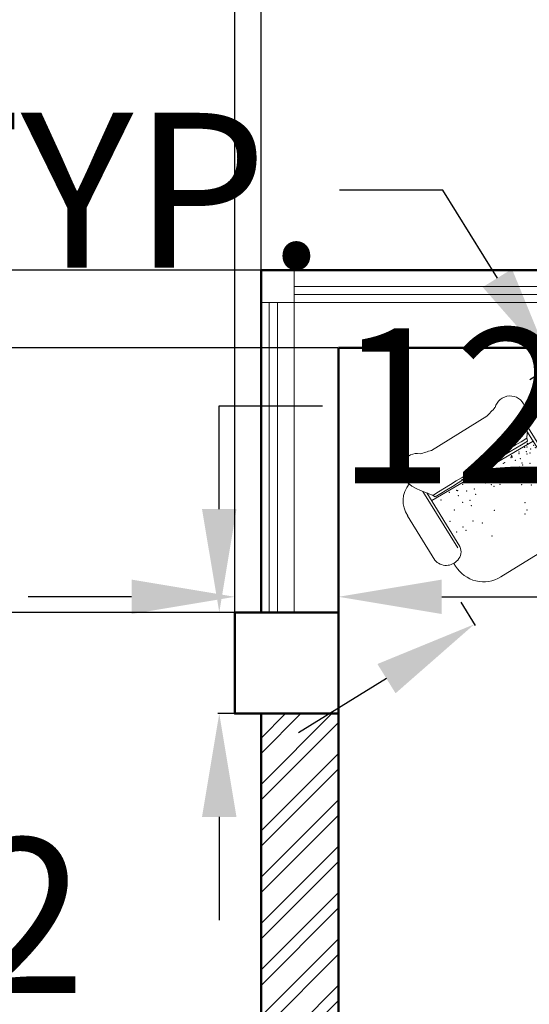
# Model space of a CAD drawing. Units: inches. Extents: x -90 to 536, y -553 to 299.
# Tile 18 of 27: x 10 to 69, y 58 to 173. Entities that reach past the tile are written whole.
import ezdxf

# ---------------------------------------------------------------- set-up
doc = ezdxf.new("R2010")
doc.units = ezdxf.units.IN
for name, color, linetype, lineweight in [('A-ANNO-DIMS', 2, 'Continuous', 18), ('A-COLS', 7, 'Continuous', 50), ('A-GLAZ', 4, 'Continuous', 18), ('A-WALL-PATT', 252, 'Continuous', 13), ('Furniture', 2, 'Continuous', 18), ('Outer Wall', 1, 'Continuous', 50)]:
    doc.layers.add(name, color=color, linetype=linetype, lineweight=lineweight)
doc.styles.get("Standard").update_dxf_attribs({"font": 'arial.ttf'})
doc.dimstyles.get("Standard").update_dxf_attribs({"dimtxt": 18, "dimasz": 12, "dimexe": 0.18, "dimexo": 0.0625, "dimgap": 0.09, "dimtad": 0, "dimtih": 1, "dimtoh": 1, "dimdec": 0, "dimzin": 0, "dimdsep": 46, "dimlunit": 3, "dimtxsty": 'Standard', "dimcen": 0.09, "dimadec": 0, "dimazin": 0, "dimtfac": 1, "dimtdec": 0, "dimtofl": 0, "dimtmove": 0, "dimatfit": 3, "dimfxl": 1, "dimtolj": 1, "dimtzin": 0, "dimarcsym": 0})

# ---------------------------------------------------------------- blocks, each defined once
blk = doc.blocks.new('A$C14440869')
for p, q in [((299.4, 786.8), (654.5, 786.8)), ((141.1, 259.3), (141.1, 621.8)), ((154.9, 258.1), (156.1, 601.9)), ((799, 258.1), (797.7, 601.9)), ((812.8, 224.7), (812.8, 621.8)), ((0, 267.1), (1, 551.8)), ((798, 537.4), (157.2, 552.6)), ((953.9, 267.1), (952.8, 551.8)), ((78.7, 198), (78.7, 179.8)), ((875.1, 196.3), (875.2, 179.8)), ((257.3, 0.1), (696.7, 0))]:
    blk.add_line(p, q)
for centre, radius, start, end in [((178, 741.7), 84.9, 46.4058, 190.9946), ((775.9, 741.7), 84.9, 349.0054, 133.5942), ((490.5, 1647.2), 881.3, 253.2515, 257.4746), ((463.3, 1647.2), 881.3, 282.5254, 286.7485), ((146, 557.8), 145.1, 108.7163, 182.3743), ((810.8, 559.8), 142.3, 356.766, 72.1434), ((234.9, -29958.2), 30532.1, 88.98134, 90.11086), ((164.3, -28909.7), 29469.6, 88.82111, 89.96326), ((79.9, 278.7), 80.7, 188.2473, 288.8842), ((90.3, 265.5), 65, 283.9696, 353.4821), ((871.6, 268.6), 73.4, 188.2144, 251.9677), ((869.8, 281.5), 85.3, 255.8372, 350.3327), ((257.8, 179.2), 179.2, 179.795, 269.795), ((696, 179.2), 179.2, 270.205, 0.205)]:
    blk.add_arc(centre, radius, start, end)
for points in [[(94.6, 725.5), (94.6, 660.2), (167.2, 599.5), (183.2, 559.8)], [(859.3, 725.5), (859.3, 660.2), (786.7, 599.5), (770.6, 553.6)]]:
    blk.add_open_spline(points, degree=3)
for p in [(261.8, 540.6), (346.3, 540.6), (358.4, 564.7), (446.9, 540.6), (467, 548.6), (656.1, 560.7), (692.1, 540.6), (752.6, 568.7), (764.7, 544.6), (201.4, 528.5), (294, 500.4), (302, 528.5), (306.1, 524.5), (346.3, 496.4), (386.5, 484.3), (446.9, 496.4), (454.9, 524.5), (487.1, 516.5), (507.2, 520.5), (531.4, 496.4), (595.7, 520.5), (603.8, 520.5), (603.8, 484.3), (647.8, 524.5), (651.8, 528.5), (656.1, 532.5), (656.1, 524.5), (659.9, 500.4), (688.3, 492.3), (696.3, 520.5), (700.3, 528.5), (732.5, 496.4), (736.6, 508.4), (740.6, 532.5), (748.6, 492.3), (752.4, 528.5), (764.7, 508.4), (788.9, 516.5), (788.9, 500.4), (233.6, 444.1), (294, 456.2), (334.2, 444.1), (378.5, 456.2), (454.9, 480.3), (479.1, 456.2), (487.1, 440.1), (519.3, 432.1), (539.4, 480.3), (543.4, 480.3), (571.6, 472.3), (659.9, 456.2), (680.2, 456.2), (684.2, 468.2), (720.2, 444.1), (792.9, 436.1), (181.3, 403.9), (326.2, 416), (692.3, 383.9), (772.5, 403.9), (181.3, 335.6), (225.6, 339.6), (290, 339.6), (418.7, 327.6), (619.9, 367.8), (663.9, 339.6), (728.3, 339.6), (772.5, 335.6), (776.8, 339.6), (229.6, 315.5), (326.2, 303.5), (583.7, 275.4), (724.3, 315.5), (551.5, 223.1), (571.6, 235.2), (334.2, 215.1)]:
    blk.add_point(p)
blk = doc.blocks.new('COL-WINDOW-PIER')
blk.add_lwpolyline([(0, 11.76), (12.04, 11.76), (12.04, 0), (0, 0)], close=True)
blk = doc.blocks.new('*D31')
at = {"layer": 'A-ANNO-DIMS', "color": 0, "lineweight": -2, "transparency": 16777216}
for p, q in [((90.45, 119.36), (100.65, 125.67)), ((100.65, 125.67), (112.65, 125.67)), ((78.67, 115.59), (80.34, 112.89)), ((61.33, 104.86), (63, 102.15)), ((52.7, 95.99), (42.5, 89.68))]:
    blk.add_line(p, q, dxfattribs=at)
at = {"layer": 'A-ANNO-DIMS', "color": 0, "transparency": 16777216}
for points in [[(89.4, 121.06), (91.5, 117.65), (80.24, 113.04)], [(51.65, 97.69), (53.76, 94.29), (62.91, 102.31)]]:
    blk.add_solid(points, dxfattribs=at)
at = {"layer": 'Defpoints', "color": 0, "transparency": 16777216}
for p in [(78.63, 115.64), (80.24, 113.04), (61.3, 104.91)]:
    blk.add_point(p, dxfattribs=at)
at = {"layer": 'A-ANNO-DIMS', "color": 0, "transparency": 16777216, "insert": (199.06, 125.67), "char_height": 18, "attachment_point": 5}
blk.add_mtext('\\A1;CHAIR 20 TYP.', dxfattribs=at)
blk = doc.blocks.new('*D32')
at = {"layer": 'A-ANNO-DIMS', "color": 0, "lineweight": -2, "transparency": 16777216}
for p, q in [((59.26, 152.75), (47.26, 152.75)), ((65.58, 142.54), (59.26, 152.75)), ((69.35, 130.76), (72.05, 132.44)), ((78.69, 115.67), (81.39, 117.34)), ((87.55, 107.05), (93.87, 96.84))]:
    blk.add_line(p, q, dxfattribs=at)
at = {"layer": 'A-ANNO-DIMS', "color": 0, "transparency": 16777216}
for points in [[(67.28, 143.6), (63.88, 141.49), (71.89, 132.34)], [(89.25, 108.1), (85.85, 105.99), (81.24, 117.25)]]:
    blk.add_solid(points, dxfattribs=at)
at = {"layer": 'Defpoints', "color": 0, "transparency": 16777216}
for p in [(71.89, 132.34), (69.29, 130.73), (78.63, 115.64)]:
    blk.add_point(p, dxfattribs=at)
at = {"layer": 'A-ANNO-DIMS', "color": 0, "transparency": 16777216, "insert": (4.21, 152.75), "char_height": 18, "attachment_point": 5}
blk.add_mtext('\\A1;18 TYP.', dxfattribs=at)
blk = doc.blocks.new('*D37')
at = {"layer": 'A-ANNO-DIMS', "color": 0, "lineweight": -2, "transparency": 16777216}
for p, q in [((23.09, 105.5), (11.09, 105.5)), ((35.09, 103.75), (35.09, 105.68)), ((47.13, 103.75), (47.13, 105.68)), ((59.13, 105.5), (71.13, 105.5))]:
    blk.add_line(p, q, dxfattribs=at)
at = {"layer": 'A-ANNO-DIMS', "color": 0, "transparency": 16777216}
for points in [[(23.09, 107.5), (23.09, 103.5), (35.09, 105.5)], [(59.13, 107.5), (59.13, 103.5), (47.13, 105.5)]]:
    blk.add_solid(points, dxfattribs=at)
at = {"layer": 'Defpoints', "color": 0, "transparency": 16777216}
for p in [(47.13, 105.5), (35.09, 103.69), (47.13, 103.69)]:
    blk.add_point(p, dxfattribs=at)
at = {"layer": 'A-ANNO-DIMS', "color": 0, "transparency": 16777216, "insert": (147.42, 105.5), "char_height": 18, "attachment_point": 5}
blk.add_mtext('\\A1;PIER 12 TYP.', dxfattribs=at)
blk = doc.blocks.new('*D38')
at = {"layer": 'A-ANNO-DIMS', "color": 0, "lineweight": -2, "transparency": 16777216}
for p, q in [((33.28, 115.69), (33.28, 127.69)), ((33.28, 127.69), (45.28, 127.69)), ((35.02, 103.69), (33.1, 103.69)), ((35.02, 91.93), (33.1, 91.93)), ((33.28, 79.93), (33.28, 67.93))]:
    blk.add_line(p, q, dxfattribs=at)
at = {"layer": 'A-ANNO-DIMS', "color": 0, "transparency": 16777216}
for points in [[(31.28, 115.69), (35.28, 115.69), (33.28, 103.69)], [(31.28, 79.93), (35.28, 79.93), (33.28, 91.93)]]:
    blk.add_solid(points, dxfattribs=at)
at = {"layer": 'Defpoints', "color": 0, "transparency": 16777216}
for p in [(33.28, 103.69), (35.09, 103.69), (35.09, 91.93)]:
    blk.add_point(p, dxfattribs=at)
at = {"layer": 'A-ANNO-DIMS', "color": 0, "transparency": 16777216, "insert": (88.33, 127.69), "char_height": 18, "attachment_point": 5}
blk.add_mtext('\\A1;12 TYP.', dxfattribs=at)
blk = doc.blocks.new('*D53')
at = {"layer": 'A-ANNO-DIMS', "color": 0, "lineweight": -2, "transparency": 16777216}
for p, q in [((35.09, 103.75), (35.09, 287.38)), ((407.13, -63.49), (407.13, 287.38)), ((47.09, 287.2), (183.7, 287.2)), ((395.13, 287.2), (258.52, 287.2))]:
    blk.add_line(p, q, dxfattribs=at)
at = {"layer": 'A-ANNO-DIMS', "color": 0, "transparency": 16777216}
for points in [[(47.09, 289.2), (47.09, 285.2), (35.09, 287.2)], [(395.13, 289.2), (395.13, 285.2), (407.13, 287.2)]]:
    blk.add_solid(points, dxfattribs=at)
at = {"layer": 'Defpoints', "color": 0, "transparency": 16777216}
for p in [(407.13, 287.2), (35.09, 103.69), (407.13, -63.55)]:
    blk.add_point(p, dxfattribs=at)
at = {"layer": 'A-ANNO-DIMS', "color": 0, "transparency": 16777216, "insert": (221.11, 287.2), "char_height": 18, "attachment_point": 5}
blk.add_mtext('\\A1;372.04', dxfattribs=at)
blk = doc.blocks.new('*D54')
at = {"layer": 'A-ANNO-DIMS', "color": 0, "lineweight": -2, "transparency": 16777216}
for p, q in [((113.07, 249.45), (-2.85, 249.45)), ((-2.67, 237.45), (-2.67, -117.77)), ((-2.67, -491.55), (-2.67, -136.34)), ((38.07, -503.55), (-2.85, -503.55))]:
    blk.add_line(p, q, dxfattribs=at)
at = {"layer": 'A-ANNO-DIMS', "color": 0, "transparency": 16777216}
for points in [[(-4.67, 237.45), (-0.67, 237.45), (-2.67, 249.45)], [(-4.67, -491.55), (-0.67, -491.55), (-2.67, -503.55)]]:
    blk.add_solid(points, dxfattribs=at)
at = {"layer": 'Defpoints', "color": 0, "transparency": 16777216}
for p in [(-2.67, 249.45), (113.13, 249.45), (38.13, -503.55)]:
    blk.add_point(p, dxfattribs=at)
at = {"layer": 'A-ANNO-DIMS', "color": 0, "transparency": 16777216, "insert": (-2.67, -127.05), "char_height": 18, "attachment_point": 5}
blk.add_mtext('\\A1;753', dxfattribs=at)
blk = doc.blocks.new('*D56')
at = {"layer": 'A-ANNO-DIMS', "color": 0, "lineweight": -2, "transparency": 16777216}
for p, q in [((47.07, 134.45), (-2.85, 134.45)), ((-2.67, 122.45), (-2.67, 77.73)), ((-2.67, 14.45), (-2.67, 59.16)), ((47.07, 2.45), (-2.85, 2.45))]:
    blk.add_line(p, q, dxfattribs=at)
at = {"layer": 'A-ANNO-DIMS', "color": 0, "transparency": 16777216}
for points in [[(-4.67, 122.45), (-0.67, 122.45), (-2.67, 134.45)], [(-4.67, 14.45), (-0.67, 14.45), (-2.67, 2.45)]]:
    blk.add_solid(points, dxfattribs=at)
at = {"layer": 'Defpoints', "color": 0, "transparency": 16777216}
for p in [(-2.67, 134.45), (47.13, 134.45), (47.13, 2.45)]:
    blk.add_point(p, dxfattribs=at)
at = {"layer": 'A-ANNO-DIMS', "color": 0, "transparency": 16777216, "insert": (-2.67, 68.45), "char_height": 18, "attachment_point": 5}
blk.add_mtext('\\A1;132', dxfattribs=at)
blk = doc.blocks.new('*D63')
at = {"layer": 'A-ANNO-DIMS', "color": 0, "lineweight": -2, "transparency": 16777216}
for p, q in [((38.13, 143.51), (38.13, 287.38)), ((110.13, 143.51), (110.13, 287.38)), ((50.13, 287.2), (61.32, 287.2)), ((98.13, 287.2), (86.95, 287.2))]:
    blk.add_line(p, q, dxfattribs=at)
at = {"layer": 'A-ANNO-DIMS', "color": 0, "transparency": 16777216}
for points in [[(50.13, 289.2), (50.13, 285.2), (38.13, 287.2)], [(98.13, 289.2), (98.13, 285.2), (110.13, 287.2)]]:
    blk.add_solid(points, dxfattribs=at)
at = {"layer": 'Defpoints', "color": 0, "transparency": 16777216}
for p in [(110.13, 287.2), (38.13, 143.45), (110.13, 143.45)]:
    blk.add_point(p, dxfattribs=at)
at = {"layer": 'A-ANNO-DIMS', "color": 0, "transparency": 16777216, "insert": (74.13, 287.2), "char_height": 18, "attachment_point": 5}
blk.add_mtext('\\A1;72', dxfattribs=at)
blk = doc.blocks.new('*D64')
at = {"layer": 'A-ANNO-DIMS', "color": 0, "lineweight": -2, "transparency": 16777216}
for p, q in [((38.07, 143.45), (-2.85, 143.45)), ((-2.67, 131.45), (-2.67, 115.69)), ((38.07, 103.69), (-2.85, 103.69)), ((-2.67, 103.69), (-2.67, 91.69)), ((-2.67, 91.69), (-14.67, 91.69))]:
    blk.add_line(p, q, dxfattribs=at)
at = {"layer": 'A-ANNO-DIMS', "color": 0, "transparency": 16777216}
for points in [[(-4.67, 131.45), (-0.67, 131.45), (-2.67, 143.45)], [(-4.67, 115.69), (-0.67, 115.69), (-2.67, 103.69)]]:
    blk.add_solid(points, dxfattribs=at)
at = {"layer": 'Defpoints', "color": 0, "transparency": 16777216}
for p in [(38.13, 143.45), (-2.67, 103.69), (38.13, 103.69)]:
    blk.add_point(p, dxfattribs=at)
at = {"layer": 'A-ANNO-DIMS', "color": 0, "transparency": 16777216, "insert": (-52.18, 91.69), "char_height": 18, "attachment_point": 5}
blk.add_mtext('\\A1;39.755', dxfattribs=at)

msp = doc.modelspace()

# ---------------------------------------------------------------- hatches: boundary and pattern name
at = {"layer": 'A-WALL-PATT'}
h = msp.add_hatch(dxfattribs=at)
h.set_pattern_fill('ANSI32', color=256, scale=0.4)
h.set_pattern_definition([(45, (-88.8105, -603.6155), (-2.694077, 2.694077), []), (45, (-87.0145, -603.6155), (-2.694077, 2.694077), [])])
h.paths.add_polyline_path([(285.1317, 246.4462), (131.1317, 246.4462), (131.1317, 237.4462), (285.1317, 237.4462)])
h.paths.add_polyline_path([(122.1317, 237.4462), (113.1317, 237.4462), (113.1317, 152.4462), (122.1317, 152.4462), (122.1317, 166.4704)])
h.paths.add_polyline_path([(303.1317, 237.4462), (294.1317, 237.4462), (294.1317, 152.4462), (303.1317, 152.4462)])
h.paths.add_polyline_path([(47.1317, 91.9277), (38.1317, 91.9277), (38.1317, -6.5538), (77.1317, -6.5538), (77.1317, 2.4462), (70.5655, 2.4462), (47.1317, 2.4462)])
h.paths.add_polyline_path([(83.052, -61.5538), (47.1317, -61.5538), (47.1317, -24.5538), (38.1317, -24.5538), (38.1317, -70.5538), (74.052, -70.5538), (74.052, -223.5538), (38.1317, -223.5538), (38.1317, -503.5538), (92.1317, -503.5538), (92.1317, -437.5538), (191.1317, -437.5538), (191.1317, -428.5538), (83.1317, -428.5538), (83.1317, -494.5538), (47.1317, -494.5538), (47.1317, -232.5538), (83.052, -232.5538), (83.052, -70.5538)])
h.paths.add_polyline_path([(407.1317, -63.5538), (381.1317, -63.5538), (381.1317, 91.9277), (372.1317, 91.9277), (372.1317, 32.8805), (372.1317, -63.5538), (306.5745, -63.5538), (237.1317, -63.5538), (237.1317, -38.5538), (233.1317, -38.5538), (233.1317, -71.5538), (398.1317, -71.5538), (398.1317, -152.5538), (233.1317, -152.5538), (233.1317, -161.5538), (398.1317, -161.5538), (398.1317, -368.5538), (233.1317, -368.5538), (233.1317, -377.5538), (407.1317, -377.5538), (407.1317, -161.5538)])
h.paths.add_polyline_path([(261.1317, -422.5538), (252.1317, -422.5538), (252.1317, -428.5538), (233.1317, -428.5538), (233.1317, -437.5538), (261.1317, -437.5538)])
h.paths.add_polyline_path([(191.1317, -368.5538), (180.1317, -368.5538), (180.1317, -335.5538), (131.5919, -335.5538), (131.5919, -344.5538), (171.1317, -344.5538), (171.1317, -392.5538), (180.1317, -392.5538), (180.1317, -377.5538), (191.1317, -377.5538)], flags=17)
h.paths.add_polyline_path([(180.1317, -223.5538), (152.1317, -223.5538), (152.1317, -227.5538), (176.1317, -227.5538), (176.1317, -335.5538), (180.1317, -335.5538)], flags=17)
h.paths.add_polyline_path([(131.5919, -335.5538), (83.1317, -335.5538), (83.1317, -339.5538), (83.1317, -392.5538), (87.1317, -392.5538), (87.1317, -339.5538), (131.5919, -339.5538)], flags=17)
h.paths.add_polyline_path([(197.1317, 2.4462), (77.1317, 2.4462), (77.1317, -1.5538), (113.1317, -1.5538), (113.1317, -71.5538), (181.1317, -71.5538), (181.1317, -67.5538), (117.1317, -67.5538), (117.1317, -1.5538), (177.1317, -1.5538), (177.1317, -37.5538), (181.1317, -37.5538), (181.1317, -1.5538), (197.1317, -1.5538)])
h.paths.add_polyline_path([(173.1317, 138.4462), (122.1317, 138.4462), (122.1317, 134.4462), (173.1317, 134.4462)])
h.paths.add_polyline_path([(213.1317, 237.4462), (209.1317, 237.4462), (209.1317, 134.4462), (233.1317, 134.4462), (233.1317, 68.8889), (233.1317, -2.5538), (237.1317, -2.5538), (237.1317, 134.4462), (258.1317, 134.4462), (258.1317, 138.4462), (213.1317, 138.4462)])

# ---------------------------------------------------------------- linework, layer by layer
at = {"layer": 'A-GLAZ'}
for p, q in [((39.0931, 139.6916), (39.0931, 103.6916)), ((41.9772, 140.6303), (78.0545, 140.6303)), ((41.9772, 139.6916), (41.9772, 103.6916))]:
    msp.add_line(p, q, dxfattribs=at)
for points in [[(38.1317, 143.4462), (41.9772, 143.4462), (41.9772, 139.6916), (38.1317, 139.6916)], [(41.9772, 139.6916), (78.0545, 139.6916), (78.0545, 141.5689), (41.9772, 141.5689)], [(38.1317, 139.6916), (40.0545, 139.6916), (40.0545, 103.6916), (38.1317, 103.6916)]]:
    msp.add_lwpolyline(points, close=True, dxfattribs=at)
at = {"layer": 'Outer Wall'}
for p, q in [((110.1317, 143.4462), (38.1317, 143.4462)), ((38.1317, 143.4462), (38.1317, 103.6916)), ((110.1317, 134.4462), (47.1317, 134.4462)), ((47.1317, 134.4462), (47.1317, 103.6916)), ((47.1317, 103.6916), (47.1317, 2.4462)), ((38.1317, 91.9277), (38.1317, -6.5538))]:
    msp.add_line(p, q, dxfattribs=at)

# ---------------------------------------------------------------- block references
at = {"layer": 'A-COLS'}
msp.add_blockref('COL-WINDOW-PIER', (35.0873, 91.9277), dxfattribs=at)
at = {"layer": 'Furniture', "xscale": 0.0212813664299499, "yscale": 0.0212813664299499, "zscale": 0.0212813664299499, "rotation": 31.75670152915393}
msp.add_blockref('A$C14440869', (61.3263, 104.927), dxfattribs=at)

# ---------------------------------------------------------------- dimensions: what is measured, and where the dimension line sits
at = {"layer": 'A-ANNO-DIMS'}
for base, p1, p2, override, picture, middle in [((407.1317, 287.2012), (35.0873, 103.6916), (407.1317, -63.5538), {"dimdec": 2, "dimlfac": 1, "dimrnd": 0, "dimzin": 0, "dimdsep": 46, "dimlunit": 2}, '*D53', (221.1095, 287.2012)), ((110.1317, 287.2012), (38.1317, 143.4462), (110.1317, 143.4462), {"dimdec": 0, "dimlfac": 1, "dimrnd": 0, "dimzin": 0, "dimdsep": 46, "dimlunit": 2}, '*D63', (74.1317, 287.2012))]:
    dim = msp.add_linear_dim(base=base, p1=p1, p2=p2, dimstyle='Standard', override=override, dxfattribs=at)
    dim.commit()
    dim.dimension.update_dxf_attribs({"geometry": picture, "text_midpoint": middle})
for base, p1, p2, override, picture, middle in [((-2.6677, 249.4462), (38.1317, -503.5538), (113.1317, 249.4462), {"dimdec": 0, "dimlfac": 1, "dimrnd": 0, "dimzin": 0, "dimdsep": 46, "dimlunit": 2}, '*D54', (-2.6677, -127.0538)), ((-2.6677, 103.6916), (38.1317, 143.4462), (38.1317, 103.6916), {"dimdec": 3, "dimlfac": 1, "dimrnd": 0, "dimzin": 0, "dimdsep": 46, "dimlunit": 2}, '*D64', (-52.182, 91.6916)), ((-2.6677, 134.4462), (47.1317, 2.4462), (47.1317, 134.4462), {"dimdec": 0, "dimlfac": 1, "dimrnd": 0, "dimzin": 0, "dimdsep": 46, "dimlunit": 2}, '*D56', (-2.6677, 68.4462))]:
    dim = msp.add_linear_dim(base=base, p1=p1, p2=p2, angle=90, dimstyle='Standard', override=override, dxfattribs=at)
    dim.commit()
    dim.dimension.update_dxf_attribs({"geometry": picture, "text_midpoint": middle})
for base, p1, p2, angle, text, picture, middle in [((71.8939, 132.3414), (78.6344, 115.6404), (69.2932, 130.7316), 121.756702, '<> TYP.', '*D32', (4.2106, 152.7484)), ((80.2442, 113.0397), (61.2964, 104.9085), (78.6344, 115.6404), 31.756702, 'CHAIR <> TYP.', '*D31', (199.0577, 125.6712)), ((33.2806, 103.6916), (35.0873, 91.9277), (35.0873, 103.6916), 90, '<> TYP.', '*D38', (88.3324, 127.6916))]:
    dim = msp.add_linear_dim(base=base, p1=p1, p2=p2, angle=angle, text=text, dimstyle='Standard', override={"dimdec": 0, "dimlfac": 1, "dimrnd": 0, "dimzin": 0, "dimdsep": 46, "dimlunit": 2}, dxfattribs=at)
    dim.commit()
    dim.dimension.update_dxf_attribs({"geometry": picture, "text_midpoint": middle})
dim = msp.add_linear_dim(base=(47.1317, 105.4983), p1=(35.0873, 103.6916), p2=(47.1317, 103.6916), text='PIER <> TYP.', dimstyle='Standard', override={"dimdec": 0, "dimlfac": 1, "dimrnd": 0, "dimzin": 0, "dimdsep": 46, "dimlunit": 2}, dxfattribs=at)
dim.commit()
dim.dimension.update_dxf_attribs({"geometry": '*D37', "text_midpoint": (147.4209, 105.4983)})

doc.saveas('drawing.dxf')
